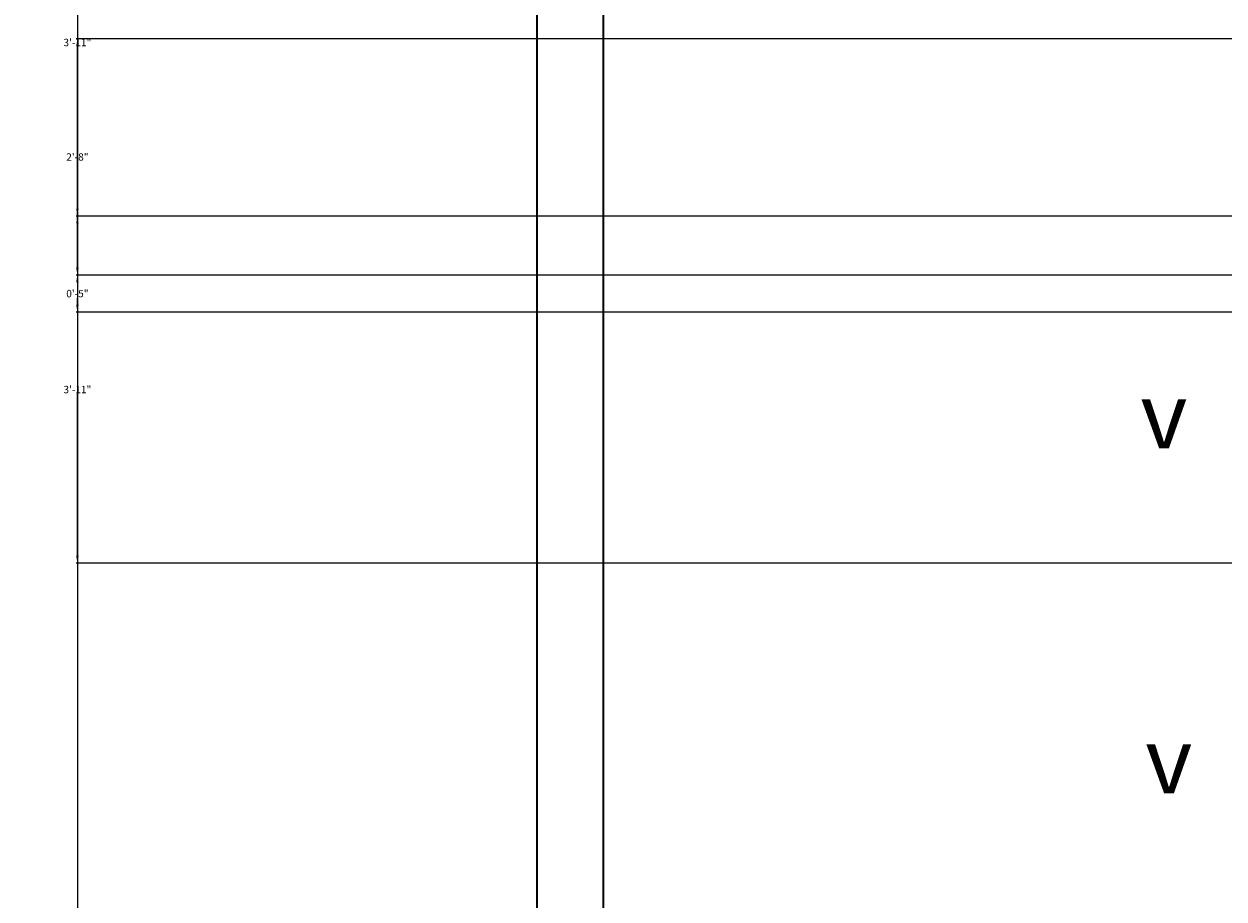
# Model space of a CAD drawing. Units: inches. Extents: x -364 to 705, y -52 to 1250.
# Tile 23 of 34: x -134 to 29, y 838 to 956. Entities that reach past the tile are written whole.
import ezdxf

# ---------------------------------------------------------------- set-up
doc = ezdxf.new("R2010")
doc.units = ezdxf.units.IN
doc.header["$MEASUREMENT"] = 0
for name, color, linetype, lineweight in [('A-ANNO-DIMS', 4, 'Continuous', 18), ('A-ANNO-IDEN', 1, 'Continuous', 18), ('C-WALL', 41, 'Continuous', 35)]:
    doc.layers.add(name, color=color, linetype=linetype, lineweight=lineweight)
doc.styles.get("Standard").update_dxf_attribs({"font": 'arial.ttf'})
doc.dimstyles.get("Standard").update_dxf_attribs({"dimtxt": 1, "dimasz": 1, "dimexe": 0.18, "dimexo": 0.0625, "dimgap": 0.09, "dimtad": 0, "dimtih": 1, "dimtoh": 1, "dimdec": 0, "dimzin": 0, "dimdsep": 46, "dimlunit": 3, "dimtxsty": 'Standard', "dimcen": 0.09, "dimadec": 0, "dimazin": 0, "dimtfac": 1, "dimtdec": 0, "dimtofl": 0, "dimtmove": 0, "dimatfit": 3, "dimfxl": 1, "dimtolj": 1, "dimtzin": 0, "dimarcsym": 0})

# ---------------------------------------------------------------- blocks, each defined once
blk = doc.blocks.new('*D19')
at = {"layer": 'A-ANNO-DIMS', "color": 0, "lineweight": -2, "transparency": 16777216}
for p, q in [((28.52, 986.11), (-248.33, 986.11)), ((-248.15, 985.11), (-248.15, 574.22)), ((-248.15, 149.87), (-248.15, 560.77)), ((28.52, 148.87), (-248.33, 148.87))]:
    blk.add_line(p, q, dxfattribs=at)
at = {"layer": 'A-ANNO-DIMS', "color": 0, "transparency": 16777216}
for points in [[(-248.32, 985.11), (-247.99, 985.11), (-248.15, 986.11)], [(-248.32, 149.87), (-247.99, 149.87), (-248.15, 148.87)]]:
    blk.add_solid(points, dxfattribs=at)
at = {"layer": 'Defpoints', "color": 0, "transparency": 16777216}
for p in [(28.58, 986.11), (-248.15, 148.87), (28.58, 148.87)]:
    blk.add_point(p, dxfattribs=at)
at = {"layer": 'A-ANNO-DIMS', "color": 0, "transparency": 16777216, "insert": (-248.15, 567.49), "char_height": 1, "attachment_point": 5}
blk.add_mtext('\\A1;{\\H13x;69\'-9"}', dxfattribs=at)
blk = doc.blocks.new('*D20')
at = {"layer": 'A-ANNO-DIMS', "color": 0, "lineweight": -2, "transparency": 16777216}
for p, q in [((28.52, 986.11), (-188.21, 986.11)), ((-188.03, 985.11), (-188.03, 917.23)), ((-188.03, 836.11), (-188.03, 904)), ((37.52, 835.11), (-188.21, 835.11))]:
    blk.add_line(p, q, dxfattribs=at)
at = {"layer": 'A-ANNO-DIMS', "color": 0, "transparency": 16777216}
for points in [[(-188.19, 985.11), (-187.86, 985.11), (-188.03, 986.11)], [(-188.19, 836.11), (-187.86, 836.11), (-188.03, 835.11)]]:
    blk.add_solid(points, dxfattribs=at)
at = {"layer": 'Defpoints', "color": 0, "transparency": 16777216}
for p in [(28.58, 986.11), (-188.03, 835.11), (37.58, 835.11)]:
    blk.add_point(p, dxfattribs=at)
at = {"layer": 'A-ANNO-DIMS', "color": 0, "transparency": 16777216, "insert": (-188.03, 910.61), "char_height": 1, "attachment_point": 5}
blk.add_mtext('\\A1;{\\H13x;12\'-7"}', dxfattribs=at)
blk = doc.blocks.new('*D76')
at = {"layer": 'A-ANNO-DIMS', "color": 0, "lineweight": -2, "transparency": 16777216}
for p, q in [((28.52, 986.11), (-126.85, 986.11)), ((-126.67, 985.11), (-126.67, 499.22)), ((-126.67, 12.11), (-126.67, 498.01)), ((28.52, 11.11), (-126.85, 11.11))]:
    blk.add_line(p, q, dxfattribs=at)
at = {"layer": 'A-ANNO-DIMS', "color": 0, "transparency": 16777216}
for points in [[(-126.84, 985.11), (-126.5, 985.11), (-126.67, 986.11)], [(-126.84, 12.11), (-126.5, 12.11), (-126.67, 11.11)]]:
    blk.add_solid(points, dxfattribs=at)
at = {"layer": 'Defpoints', "color": 0, "transparency": 16777216}
for p in [(-126.67, 986.11), (28.58, 986.11), (28.58, 11.11)]:
    blk.add_point(p, dxfattribs=at)
at = {"layer": 'A-ANNO-DIMS', "color": 0, "transparency": 16777216, "insert": (-126.67, 498.61), "char_height": 1, "attachment_point": 5}
blk.add_mtext('\\A1;81\'-3"', dxfattribs=at)
blk = doc.blocks.new('*D93')
at = {"layer": 'A-ANNO-DIMS', "color": 0, "lineweight": -2, "transparency": 16777216}
for p, q in [((37.52, 977.11), (-126.85, 977.11)), ((-126.67, 976.11), (-126.67, 954.22)), ((-126.67, 931.11), (-126.67, 953.01)), ((37.52, 930.11), (-126.85, 930.11))]:
    blk.add_line(p, q, dxfattribs=at)
at = {"layer": 'A-ANNO-DIMS', "color": 0, "transparency": 16777216}
for points in [[(-126.84, 976.11), (-126.5, 976.11), (-126.67, 977.11)], [(-126.84, 931.11), (-126.5, 931.11), (-126.67, 930.11)]]:
    blk.add_solid(points, dxfattribs=at)
at = {"layer": 'Defpoints', "color": 0, "transparency": 16777216}
for p in [(37.58, 977.11), (-126.67, 930.11), (37.58, 930.11)]:
    blk.add_point(p, dxfattribs=at)
at = {"layer": 'A-ANNO-DIMS', "color": 0, "transparency": 16777216, "insert": (-126.67, 953.61), "char_height": 1, "attachment_point": 5}
blk.add_mtext('\\A1;3\'-11"', dxfattribs=at)
blk = doc.blocks.new('*D94')
at = {"layer": 'A-ANNO-DIMS', "color": 0, "lineweight": -2, "transparency": 16777216}
for p, q in [((37.52, 930.11), (-126.85, 930.11)), ((-126.67, 929.11), (-126.67, 907.22)), ((-126.67, 884.11), (-126.67, 906.01)), ((37.52, 883.11), (-126.85, 883.11))]:
    blk.add_line(p, q, dxfattribs=at)
at = {"layer": 'A-ANNO-DIMS', "color": 0, "transparency": 16777216}
for points in [[(-126.84, 929.11), (-126.5, 929.11), (-126.67, 930.11)], [(-126.84, 884.11), (-126.5, 884.11), (-126.67, 883.11)]]:
    blk.add_solid(points, dxfattribs=at)
at = {"layer": 'Defpoints', "color": 0, "transparency": 16777216}
for p in [(37.58, 930.11), (-126.67, 883.11), (37.58, 883.11)]:
    blk.add_point(p, dxfattribs=at)
at = {"layer": 'A-ANNO-DIMS', "color": 0, "transparency": 16777216, "insert": (-126.67, 906.61), "char_height": 1, "attachment_point": 5}
blk.add_mtext('\\A1;3\'-11"', dxfattribs=at)
blk = doc.blocks.new('*D103')
at = {"layer": 'A-ANNO-DIMS', "color": 0, "lineweight": -2, "transparency": 16777216}
for p, q in [((193.52, 954.1), (-126.85, 954.1)), ((-126.67, 953.1), (-126.67, 938.71)), ((-126.67, 923.11), (-126.67, 937.51)), ((193.52, 922.11), (-126.85, 922.11))]:
    blk.add_line(p, q, dxfattribs=at)
at = {"layer": 'A-ANNO-DIMS', "color": 0, "transparency": 16777216}
for points in [[(-126.84, 953.1), (-126.5, 953.1), (-126.67, 954.1)], [(-126.84, 923.11), (-126.5, 923.11), (-126.67, 922.11)]]:
    blk.add_solid(points, dxfattribs=at)
at = {"layer": 'Defpoints', "color": 0, "transparency": 16777216}
for p in [(-126.67, 954.1), (193.58, 954.1), (193.58, 922.11)]:
    blk.add_point(p, dxfattribs=at)
at = {"layer": 'A-ANNO-DIMS', "color": 0, "transparency": 16777216, "insert": (-126.67, 938.11), "char_height": 1, "attachment_point": 5}
blk.add_mtext('\\A1;2\'-8"', dxfattribs=at)
blk = doc.blocks.new('*D104')
at = {"layer": 'A-ANNO-DIMS', "color": 0, "lineweight": -2, "transparency": 16777216}
for p, q in [((193.52, 922.11), (-126.85, 922.11)), ((-126.67, 921.11), (-126.67, 920.22)), ((-126.67, 918.11), (-126.67, 919.01)), ((193.52, 917.11), (-126.85, 917.11))]:
    blk.add_line(p, q, dxfattribs=at)
at = {"layer": 'A-ANNO-DIMS', "color": 0, "transparency": 16777216}
for points in [[(-126.84, 921.11), (-126.5, 921.11), (-126.67, 922.11)], [(-126.84, 918.11), (-126.5, 918.11), (-126.67, 917.11)]]:
    blk.add_solid(points, dxfattribs=at)
at = {"layer": 'Defpoints', "color": 0, "transparency": 16777216}
for p in [(-126.67, 922.11), (193.58, 922.11), (193.58, 917.11)]:
    blk.add_point(p, dxfattribs=at)
at = {"layer": 'A-ANNO-DIMS', "color": 0, "transparency": 16777216, "insert": (-126.67, 919.61), "char_height": 1, "attachment_point": 5}
blk.add_mtext('\\A1;0\'-5"', dxfattribs=at)

msp = doc.modelspace()

# ---------------------------------------------------------------- linework, layer by layer
at = {"layer": 'C-WALL'}
for p, q in [((-64.42, 11.11), (-64.42, 1079.11)), ((-55.42, 11.11), (-55.42, 1070.11))]:
    msp.add_line(p, q, dxfattribs=at)

# ---------------------------------------------------------------- texts
at = {"layer": 'A-ANNO-IDEN', "char_height": 9, "attachment_point": 1}
for insert in [(17.24, 907.64), (17.91, 860.91)]:
    msp.add_mtext_dynamic_manual_height_columns('v', width=10.6887, gutter_width=1, heights=[0], dxfattribs=dict(at, insert=insert))

# ---------------------------------------------------------------- dimensions: what is measured, and where the dimension line sits
at = {"layer": 'A-ANNO-DIMS'}
dim = msp.add_linear_dim(base=(-248.15, 148.87), p1=(28.58, 986.11), p2=(28.58, 148.87), angle=90, text='{\\H13x;<>}', dimstyle='Standard', override={"dimclrd": 0, "dimclre": 0, "dimclrt": 0}, dxfattribs=at)
dim.commit()
dim.dimension.update_dxf_attribs({"geometry": '*D19', "text_midpoint": (-248.15, 567.49)})
dim = msp.add_linear_dim(base=(-188.03, 835.11), p1=(28.58, 986.11), p2=(37.58, 835.11), angle=90, text='{\\H13x;<>}', dimstyle='Standard', override={"dimclrd": 0, "dimclre": 0, "dimclrt": 0}, dxfattribs=at)
dim.commit()
dim.dimension.update_dxf_attribs({"geometry": '*D20', "text_midpoint": (-188.03, 910.61), "dimtype": 160})
for base, p1, p2, picture, middle in [((-126.67, 986.11), (28.58, 11.11), (28.58, 986.11), '*D76', (-126.67, 498.61)), ((-126.67, 930.11), (37.58, 977.11), (37.58, 930.11), '*D93', (-126.67, 953.61)), ((-126.67, 954.1), (193.58, 922.11), (193.58, 954.1), '*D103', (-126.67, 938.11)), ((-126.67, 883.11), (37.58, 930.11), (37.58, 883.11), '*D94', (-126.67, 906.61)), ((-126.67, 922.11), (193.58, 917.11), (193.58, 922.11), '*D104', (-126.67, 919.61))]:
    dim = msp.add_linear_dim(base=base, p1=p1, p2=p2, angle=90, dimstyle='Standard', override={"dimdec": 1, "dimlfac": 1, "dimrnd": 0, "dimzin": 1, "dimdsep": 46, "dimlunit": 4, "dimfrac": 2}, dxfattribs=at)
    dim.commit()
    dim.dimension.update_dxf_attribs({"geometry": picture, "text_midpoint": middle})

doc.saveas('drawing.dxf')
